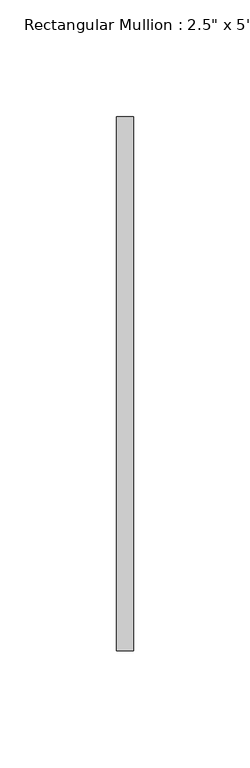
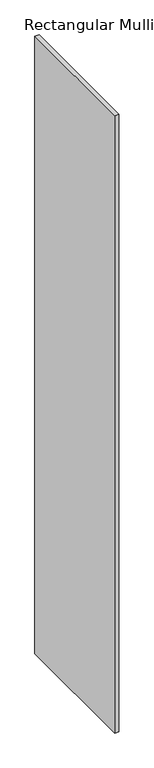
"""IFC4 building model written with IfcOpenShell, lengths in millimetres: member geometry."""

from ifc_helpers import new_model, si_unit, frame, origin, place, context, project, spatial, polyline, outline, extrude, source, transform, mapped, element, save


def member_2d61f393(model_context):
    return source(origin(), model_context, "Body", "SweptSolid", [
        extrude(outline(polyline([(0.0, 114.3), (0.0, -114.3), (-7.239, -114.3), (-7.239, 114.3), (0.0, 114.3)])), frame((0.0, 0.0, -1081.3415), z_axis=(0.0, 0.0, 1.0), x_axis=(1.0, 0.0, 0.0)), (0.0, 0.0, 1.0), 1081.3415),
    ])


if __name__ == "__main__":
    model = new_model("IFC4")
    model_context = context("Model", 3, world=origin())
    ifc_project = project(units=[si_unit("LENGTHUNIT", "METRE", prefix="MILLI")], contexts=[model_context])
    site = spatial("IfcSite", under=ifc_project)
    building = spatial("IfcBuilding", under=site)
    placement = place(None, origin())
    member_shape = member_2d61f393(model_context)
    element("IfcMember", 1, ObjectType="Rectangular Mullion : 2.5\" x 5\" rectangular", at=placement, inside=building, context=model_context, shape_type="MappedRepresentation", body=[
        mapped(member_shape, transform((0.0, 0.0, 0.0), x_axis=(1.0, 0.0, 0.0), y_axis=(0.0, 1.0, 0.0), z_axis=(0.0, 0.0, 1.0))),
    ])
    save(model, "model.ifc")

# Revit data of these elements
# Type "Rectangular Mullion : 2.5\" x 5\" rectangular"
#   built-in parameter 1007304 = 0.75 (stored number, unit not read)
#   built-in parameter 1007301 = 0.011875 (stored number, unit not read)
#   built-in parameter 1007300 = 0.011875 (stored number, unit not read)
# Element 1 (IfcMember, "Rectangular Mullion : 2.5\" x 5\" rectangular")
#   Materials on its faces: "WINDOW GLASS MATERIAL"
# Materials
#   "WINDOW GLASS MATERIAL": class "Generic", colour RGB 120 120 120, transparency 0, Cost = 0
